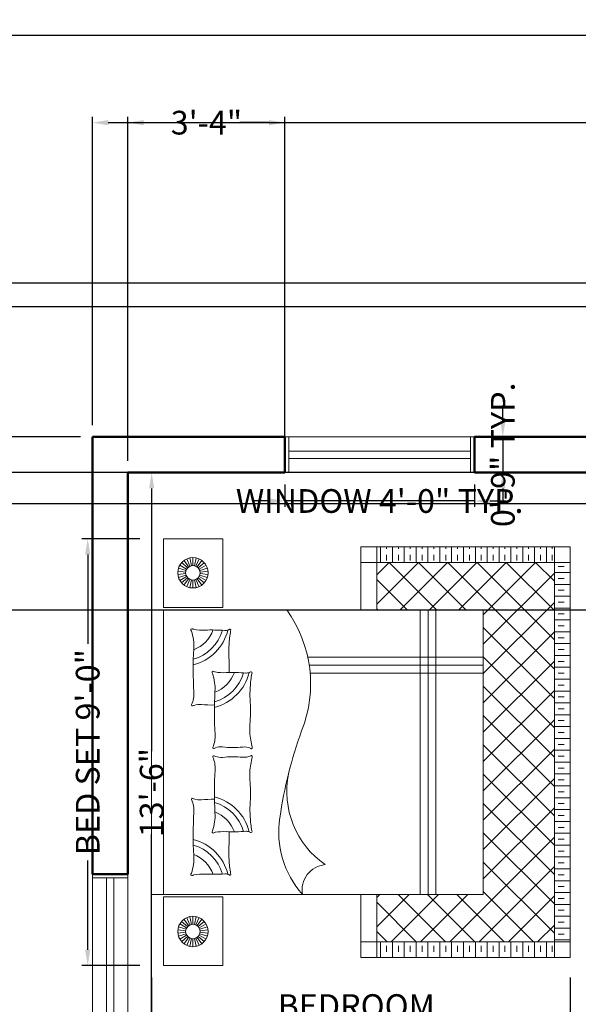
# Model space of a CAD drawing. Units: inches. Extents: x 6704 to 7574, y 11759 to 12617.
# Tile 6 of 8: x 6900 to 7041, y 12368 to 12617. Entities that reach past the tile are written whole.
import ezdxf

# ---------------------------------------------------------------- set-up
doc = ezdxf.new("R2010")
doc.units = ezdxf.units.IN
doc.header["$MEASUREMENT"] = 0
for name, color, linetype, lineweight in [('A-AREA-IDEN', 7, 'Continuous', 18), ('A-FURN', 8, 'Continuous', 18), ('C-PROP', 7, 'Continuous', 30), ('WALL', 7, 'Continuous', 50), ('WINDOW', 2, 'Continuous', 20), ('YQ_DIM', 3, 'Continuous', 18)]:
    doc.layers.add(name, color=color, linetype=linetype, lineweight=lineweight)
doc.styles.get("Standard").update_dxf_attribs({"font": 'arial.ttf'})
doc.styles.add('YQ_DIM', font='SUPEROS.SHX', dxfattribs={"width": 0.8, "bigfont": 'HZDX.SHX'})
doc.dimstyles.new('yqi0', dxfattribs={"dimscale": 0, "dimtxt": 6, "dimasz": 4, "dimexe": 1.5, "dimexo": 3, "dimgap": 0.5, "dimtad": 0, "dimdsep": 46, "dimlunit": 4, "dimtxsty": 'Standard', "dimcen": 0, "dimclrd": 256, "dimclre": 256, "dimclrt": 7, "dimadec": 1, "dimazin": 2, "dimtfac": 1, "dimtix": 1, "dimtmove": 2, "dimatfit": 2, "dimfxl": 1, "dimtolj": 1, "dimtzin": 0, "dimarcsym": 0})

# ---------------------------------------------------------------- blocks, each defined once
blk = doc.blocks.new('*D2')
at = {"layer": 'Defpoints', "color": 0, "transparency": 16777216}
for p in [(7311.07, 12612.93), (6879.07, 12550.26), (7311.07, 12550.26)]:
    blk.add_point(p, dxfattribs=at)
at = {"layer": 'YQ_DIM', "color": 0, "lineweight": -2, "transparency": 16777216}
for p, q in [((6879.07, 12553.26), (6879.07, 12614.43)), ((7311.07, 12553.26), (7311.07, 12614.43)), ((6883.07, 12612.93), (7089.48, 12612.93)), ((7307.07, 12612.93), (7100.66, 12612.93))]:
    blk.add_line(p, q, dxfattribs=at)
at = {"layer": 'YQ_DIM', "color": 0, "transparency": 16777216}
for points in [[(6883.07, 12613.6), (6883.07, 12612.27), (6879.07, 12612.93)], [(7307.07, 12613.6), (7307.07, 12612.27), (7311.07, 12612.93)]]:
    blk.add_solid(points, dxfattribs=at)
at = {"layer": 'YQ_DIM', "color": 0, "transparency": 16777216, "insert": (7095.07, 12612.93), "char_height": 6, "attachment_point": 5}
blk.add_mtext("\\A1;36'", dxfattribs=at)
blk = doc.blocks.new('*D4')
at = {"layer": 'Defpoints', "color": 0, "transparency": 16777216}
for p in [(6927.07, 12502.26), (6927.07, 12340.26), (6933.07, 12340.26)]:
    blk.add_point(p, dxfattribs=at)
at = {"layer": 'YQ_DIM', "color": 0, "lineweight": -2, "transparency": 16777216}
for p, q in [((6930.07, 12502.26), (6934.57, 12502.26)), ((6933.07, 12498.26), (6933.07, 12431.78)), ((6933.07, 12344.26), (6933.07, 12410.73)), ((6930.07, 12340.26), (6934.57, 12340.26))]:
    blk.add_line(p, q, dxfattribs=at)
at = {"layer": 'YQ_DIM', "color": 0, "transparency": 16777216}
for points in [[(6932.41, 12498.26), (6933.74, 12498.26), (6933.07, 12502.26)], [(6932.41, 12344.26), (6933.74, 12344.26), (6933.07, 12340.26)]]:
    blk.add_solid(points, dxfattribs=at)
at = {"layer": 'YQ_DIM', "color": 0, "transparency": 16777216, "insert": (6933.07, 12421.26), "char_height": 6, "attachment_point": 5, "rotation": 90}
blk.add_mtext('\\A1;13\'-6"', dxfattribs=at)
blk = doc.blocks.new('WD_00_X1')
for p, q in [((-0.5, 0.5), (0.5, 0.5)), ((-0.48, 0.5), (-0.48, -0.5)), ((0.48, 0.5), (0.48, -0.5)), ((0.48, 0.1), (-0.48, 0.1)), ((0.48, -0.1), (-0.48, -0.1)), ((-0.5, -0.5), (0.5, -0.5))]:
    blk.add_line(p, q)
blk = doc.blocks.new('BED')
h = blk.add_hatch()
h.set_pattern_fill('TRANS', color=256, scale=12, style=0)
h.set_pattern_definition([(360, (4433.967, -9715.0492), (1e-15, 3), []), (360, (4433.967, -9713.5492), (1e-15, 3), [1.5, -1.5])])
h.paths.add_polyline_path([(48, -103), (52, -103), (52, -58), (48, -58)])
h.paths.add_polyline_path([(-48, -58), (-52, -58), (-52, -103), (-48, -103)])
h = blk.add_hatch()
h.set_pattern_fill('ANSI37', color=256, scale=42, angle=-90, style=0)
h.set_pattern_definition([(315, (7787.1367, 4477.8466), (3.7123106, 3.7123106), []), (45, (7787.1367, 4477.8466), (-3.7123106, 3.7123106), [])])
h.paths.add_polyline_path([(-36, -85), (-36, -58), (-48, -58), (-48, -103), (48, -103), (48, -58), (36, -58), (36, -85)])
h = blk.add_hatch()
h.set_pattern_fill('TRANS', color=256, scale=12, angle=-90, style=0)
h.set_pattern_definition([(270, (4433.967, -9715.0492), (3, -1e-15), []), (270, (4435.467, -9715.0492), (3, -1e-15), [1.5, -1.5])])
h.paths.add_polyline_path([(48, -107), (48, -103), (-48, -103), (-48, -107)])
for p, q in [((-36, -1), (36, -1)), ((-36, -85), (-36, -1)), ((36, -1), (36, -85)), ((-54, -4), (-54, -19)), ((-36.64, -4), (-54, -4)), ((-36.64, -4), (-36.64, -19)), ((-36, -4), (36, -4)), ((36.64, -4), (36.64, -19)), ((36.64, -4), (54, -4)), ((54, -4), (54, -19)), ((-47.07, -10.7), (-48.9, -9.89)), ((-46.88, -10.37), (-48.5, -9.2)), ((-46.62, -10.08), (-47.96, -8.6)), ((-46.31, -9.86), (-47.31, -8.13)), ((-45.96, -9.7), (-46.58, -7.8)), ((-45.58, -9.62), (-45.8, -7.63)), ((-45.2, -9.62), (-45, -7.63)), ((-44.82, -9.7), (-44.21, -7.79)), ((-44.47, -9.85), (-43.48, -8.12)), ((-44.16, -10.08), (-42.83, -8.59)), ((-43.9, -10.36), (-42.29, -9.18)), ((-43.71, -10.7), (-41.89, -9.88)), ((43.71, -10.7), (41.89, -9.88)), ((43.9, -10.36), (42.29, -9.18)), ((44.16, -10.08), (42.83, -8.59)), ((44.47, -9.85), (43.48, -8.12)), ((44.82, -9.7), (44.21, -7.79)), ((45.2, -9.62), (45, -7.63)), ((45.58, -9.62), (45.8, -7.63)), ((45.96, -9.7), (46.58, -7.8)), ((46.31, -9.86), (47.31, -8.13)), ((46.62, -10.08), (47.96, -8.6)), ((46.88, -10.37), (48.5, -9.2)), ((47.07, -10.7), (48.9, -9.89)), ((-47.23, -11.45), (-49.23, -11.45)), ((-47.19, -11.07), (-49.14, -10.66)), ((-47.19, -11.83), (-49.14, -12.25)), ((-47.07, -12.2), (-48.89, -13.01)), ((-43.71, -12.19), (-41.88, -13)), ((-43.59, -11.06), (-41.64, -10.64)), ((-43.59, -11.83), (-41.63, -12.24)), ((-43.55, -11.44), (-41.55, -11.44)), ((43.55, -11.44), (41.55, -11.44)), ((43.59, -11.83), (41.63, -12.24)), ((43.59, -11.06), (41.64, -10.64)), ((43.71, -12.19), (41.88, -13)), ((47.07, -12.2), (48.89, -13.01)), ((47.19, -11.07), (49.14, -10.66)), ((47.19, -11.83), (49.14, -12.25)), ((47.23, -11.45), (49.23, -11.45)), ((-46.87, -12.53), (-48.49, -13.71)), ((-46.62, -12.81), (-47.95, -14.3)), ((-46.3, -13.04), (-47.3, -14.77)), ((-45.95, -13.2), (-46.57, -15.1)), ((-45.58, -13.27), (-45.78, -15.26)), ((-45.19, -13.27), (-44.98, -15.26)), ((-44.82, -13.19), (-44.2, -15.09)), ((-44.47, -13.04), (-43.46, -14.77)), ((-44.16, -12.81), (-42.82, -14.29)), ((-43.9, -12.52), (-42.28, -13.7)), ((43.9, -12.52), (42.28, -13.7)), ((44.16, -12.81), (42.82, -14.29)), ((44.47, -13.04), (43.46, -14.77)), ((44.82, -13.19), (44.2, -15.09)), ((45.19, -13.27), (44.98, -15.26)), ((45.58, -13.27), (45.78, -15.26)), ((45.95, -13.2), (46.57, -15.1)), ((46.3, -13.04), (47.3, -14.77)), ((46.62, -12.81), (47.95, -14.3)), ((46.87, -12.53), (48.49, -13.71)), ((-36.64, -19), (-54, -19)), ((36.64, -19), (54, -19)), ((20, -85), (20, -41.14)), ((22, -85), (22, -40.91)), ((24, -85), (24, -40.55)), ((-52, -54), (-52, -107)), ((-52, -54), (-36, -54)), ((-48, -54), (-48, -107)), ((36, -54), (52, -54)), ((48, -54), (48, -107)), ((52, -54), (52, -107)), ((-52, -58), (-36, -58)), ((36, -58), (52, -58)), ((36, -69), (-36, -69)), ((36, -71), (-36, -71)), ((36, -73), (-36, -73)), ((36, -85), (-36, -85)), ((-52, -103), (52, -103)), ((-52, -107), (52, -107))]:
    blk.add_line(p, q)
for centre, radius in [((-45.39, -11.45), 3.84), ((-45.39, -11.45), 1.84), ((45.39, -11.45), 3.84), ((45.39, -11.45), 1.84)]:
    blk.add_circle(centre, radius)
for centre, radius, start, end in [((-30.92, -11.24), 0.328, 35.8976, 208.6272), ((-42.38, -17.5), 12.73, 27.1629, 28.6272), ((-44.37, -13.89), 13.5, 357.4804, 9.3956), ((-33.8, -8.61), 8.46, 289.8695, 338.9843), ((-33.8, -8.61), 12.06, 283.8498, 346.0842), ((-33.8, -8.61), 10.71, 286.0319, 344.1205), ((-26.84, 0.13), 11.82, 251.1782, 273.3982), ((-20.92, -99.64), 88.13, 86.2964, 93.3982), ((-14.79, -4.98), 6.73, 266.2964, 294.303), ((-8.24, -13.16), 3.86, 159.0146, 186.273), ((-11.92, -11.33), 0.242, 335.7259, 114.303), ((-5.69, -14.14), 6.59, 155.7259, 159.0146), ((11.92, -11.33), 0.242, 65.697, 204.2741), ((5.69, -14.14), 6.59, 20.9854, 24.2741), ((8.24, -13.16), 3.86, 353.727, 20.9854), ((14.79, -4.98), 6.73, 245.697, 273.7036), ((20.92, -99.64), 88.13, 86.6018, 93.7036), ((33.8, -8.61), 12.06, 193.9158, 256.1502), ((33.8, -8.61), 10.71, 195.8795, 253.9681), ((33.8, -8.61), 8.46, 201.0157, 250.1305), ((26.84, 0.13), 11.82, 266.6018, 288.8218), ((30.92, -11.24), 0.328, 331.3728, 144.1024), ((44.37, -13.89), 13.5, 170.6044, 182.5196), ((42.38, -17.5), 12.73, 151.3728, 152.8371), ((10.15, -16.29), 41.07, 177.4804, 184.5075), ((-36.64, -16.28), 24.71, 358.5721, 6.273), ((36.64, -16.28), 24.71, 173.727, 181.4279), ((-10.15, -16.29), 41.07, 355.4925, 2.5196), ((-20.16, -16.62), 0.328, 35.8976, 208.6272), ((-31.62, -22.87), 12.73, 27.1629, 28.6272), ((-33.61, -19.26), 13.5, 357.4804, 9.3956), ((-23.04, -13.99), 8.46, 289.8695, 338.9843), ((-23.04, -13.99), 12.06, 283.8498, 346.0842), ((-23.04, -13.99), 10.71, 286.0319, 344.1205), ((-16.08, -5.24), 11.82, 251.1782, 273.3982), ((-10.15, -105.01), 88.13, 86.2964, 93.3982), ((-4.03, -10.35), 6.73, 266.2964, 294.303), ((2.52, -18.53), 3.86, 159.0146, 186.273), ((-1.16, -16.7), 0.242, 335.7259, 114.303), ((5.07, -19.51), 6.59, 155.7259, 159.0146), ((1.16, -16.7), 0.242, 65.697, 204.2741), ((-5.07, -19.51), 6.59, 20.9854, 24.2741), ((-2.52, -18.53), 3.86, 353.727, 20.9854), ((4.03, -10.35), 6.73, 245.697, 273.7036), ((10.15, -105.01), 88.13, 86.6018, 93.7036), ((23.04, -13.99), 12.06, 193.9158, 256.1502), ((23.04, -13.99), 10.71, 195.8795, 253.9681), ((23.04, -13.99), 8.46, 201.0157, 250.1305), ((16.08, -5.24), 11.82, 266.6018, 288.8218), ((20.16, -16.62), 0.328, 331.3728, 144.1024), ((33.61, -19.26), 13.5, 170.6044, 182.5196), ((31.62, -22.87), 12.73, 151.3728, 152.8371), ((-32.67, -19.67), 1.88, 339.2246, 4.5075), ((20.91, -21.66), 41.07, 177.4804, 184.5075), ((-25.88, -21.66), 24.71, 354.3784, 6.273), ((25.88, -21.66), 24.71, 173.727, 185.6216), ((-20.91, -21.66), 41.07, 355.4925, 2.5196), ((32.67, -19.67), 1.88, 175.4925, 200.7754), ((-30.88, -20.82), 0.25, 147.6219, 311.9343), ((-32.72, -19.65), 1.93, 327.6219, 339.2246), ((-25.16, -53.53), 33, 93.5164, 99.6766), ((-25.27, -51.86), 31.33, 86.4836, 93.5164), ((-21.12, 15.68), 36.34, 266.4836, 271.5234), ((21.12, 15.68), 36.34, 268.4766, 273.5164), ((25.27, -51.86), 31.33, 86.4836, 93.5164), ((25.16, -53.53), 33, 80.3234, 86.4836), ((30.88, -20.82), 0.25, 228.0657, 32.3781), ((32.72, -19.65), 1.93, 200.7754, 212.3781), ((-21.91, -25.04), 1.88, 339.2246, 4.5075), ((2.55, -24.46), 3.86, 174.3784, 204.7617), ((-2.55, -24.46), 3.86, 335.2383, 5.6216), ((21.91, -25.04), 1.88, 175.4925, 200.7754), ((-20.12, -26.19), 0.25, 147.6219, 311.9343), ((-21.96, -25.02), 1.93, 327.6219, 339.2246), ((-14.4, -58.9), 33, 93.5164, 99.6766), ((-14.51, -57.23), 31.33, 86.4836, 93.5164), ((-10.35, 10.3), 36.34, 266.4836, 275.306), ((-5.78, -38.98), 13.15, 77.9645, 95.306), ((2.5, -0.17), 26.53, 257.9645, 261.9243), ((-1.09, -26.25), 0.228, 231.9005, 52.8902), ((1.09, -26.25), 0.228, 127.1098, 308.0995), ((-2.5, -0.17), 26.53, 278.0757, 282.0355), ((5.78, -38.98), 13.15, 84.694, 102.0355), ((10.35, 10.3), 36.34, 264.694, 273.5164), ((14.51, -57.23), 31.33, 86.4836, 93.5164), ((14.4, -58.9), 33, 80.3234, 86.4836), ((20.12, -26.19), 0.25, 228.0657, 32.3781), ((21.96, -25.02), 1.93, 200.7754, 212.3781), ((-20.27, -56.85), 23.66, 81.0857, 131.6581), ((-32.56, -143.87), 111.55, 70.0977, 81.7735), ((-9.91, -57.83), 22.61, 78.6456, 145.1521), ((17.27, -9.21), 32.05, 248.2778, 305.7663), ((-34.97, -45.63), 6.55, 6.3172, 99.0807)]:
    blk.add_arc(centre, radius, start, end)
blk = doc.blocks.new('*D31')
at = {"layer": 'Defpoints', "color": 0, "transparency": 16777216}
for p in [(6966.82, 12502.26), (7014.82, 12502.26), (6966.82, 12495.06)]:
    blk.add_point(p, dxfattribs=at)
at = {"layer": 'YQ_DIM', "lineweight": -2, "transparency": 16777216}
for p, q in [((6966.82, 12499.26), (6966.82, 12493.56)), ((7014.82, 12499.26), (7014.82, 12493.56)), ((6962.82, 12495.06), (6958.82, 12495.06)), ((7014.82, 12495.06), (6966.82, 12495.06)), ((7018.82, 12495.06), (7022.82, 12495.06))]:
    blk.add_line(p, q, dxfattribs=at)
at = {"layer": 'YQ_DIM', "transparency": 16777216}
for points in [[(6962.82, 12495.72), (6962.82, 12494.39), (6966.82, 12495.06)], [(7018.82, 12495.72), (7018.82, 12494.39), (7014.82, 12495.06)]]:
    blk.add_solid(points, dxfattribs=at)
at = {"layer": 'YQ_DIM', "color": 7, "transparency": 16777216, "insert": (6990.82, 12495.06), "char_height": 6, "attachment_point": 5}
blk.add_mtext('\\A1;WINDOW 4\'-0" TYP.', dxfattribs=at)
blk = doc.blocks.new('*D32')
at = {"layer": 'Defpoints', "color": 0, "transparency": 16777216}
for p in [(7014.82, 12511.26), (7014.82, 12502.26), (7022.02, 12502.26)]:
    blk.add_point(p, dxfattribs=at)
at = {"layer": 'YQ_DIM', "lineweight": -2, "transparency": 16777216}
for p, q in [((7022.02, 12515.26), (7022.02, 12519.26)), ((7017.82, 12511.26), (7023.52, 12511.26)), ((7022.02, 12511.26), (7022.02, 12502.26)), ((7017.82, 12502.26), (7023.52, 12502.26)), ((7022.02, 12498.26), (7022.02, 12494.26))]:
    blk.add_line(p, q, dxfattribs=at)
at = {"layer": 'YQ_DIM', "transparency": 16777216}
for points in [[(7021.36, 12515.26), (7022.69, 12515.26), (7022.02, 12511.26)], [(7021.36, 12498.26), (7022.69, 12498.26), (7022.02, 12502.26)]]:
    blk.add_solid(points, dxfattribs=at)
at = {"layer": 'YQ_DIM', "color": 7, "transparency": 16777216, "insert": (7022.02, 12506.76), "char_height": 6, "attachment_point": 5, "rotation": 90}
blk.add_mtext('\\A1;0\'-9" TYP.', dxfattribs=at)
blk = doc.blocks.new('*D39')
at = {"layer": 'Defpoints', "color": 0, "transparency": 16777216}
for p in [(6916.87, 12485.5), (6933.07, 12485.5), (6933.07, 12377.5)]:
    blk.add_point(p, dxfattribs=at)
at = {"layer": 'YQ_DIM', "lineweight": -2, "transparency": 16777216}
for p, q in [((6930.07, 12485.5), (6915.37, 12485.5)), ((6916.87, 12481.5), (6916.87, 12458.93)), ((6916.87, 12381.5), (6916.87, 12404.06)), ((6930.07, 12377.5), (6915.37, 12377.5))]:
    blk.add_line(p, q, dxfattribs=at)
at = {"layer": 'YQ_DIM', "transparency": 16777216}
for points in [[(6916.21, 12481.5), (6917.54, 12481.5), (6916.87, 12485.5)], [(6916.21, 12381.5), (6917.54, 12381.5), (6916.87, 12377.5)]]:
    blk.add_solid(points, dxfattribs=at)
at = {"layer": 'YQ_DIM', "color": 7, "transparency": 16777216, "insert": (6916.87, 12431.5), "char_height": 6, "attachment_point": 5, "rotation": 90}
blk.add_mtext('\\A1;BED SET 9\'-0"', dxfattribs=at)
blk = doc.blocks.new('*D40')
at = {"layer": 'Defpoints', "color": 0, "transparency": 16777216}
for p in [(6933.07, 12377.5), (7039.07, 12377.5), (6933.07, 12361.3)]:
    blk.add_point(p, dxfattribs=at)
at = {"layer": 'YQ_DIM', "lineweight": -2, "transparency": 16777216}
for p, q in [((6933.07, 12374.5), (6933.07, 12359.8)), ((7039.07, 12374.5), (7039.07, 12359.8)), ((6937.07, 12361.3), (6975.26, 12361.3)), ((7035.07, 12361.3), (6996.88, 12361.3))]:
    blk.add_line(p, q, dxfattribs=at)
at = {"layer": 'YQ_DIM', "transparency": 16777216}
for points in [[(6937.07, 12361.96), (6937.07, 12360.63), (6933.07, 12361.3)], [(7035.07, 12361.96), (7035.07, 12360.63), (7039.07, 12361.3)]]:
    blk.add_solid(points, dxfattribs=at)
at = {"layer": 'YQ_DIM', "color": 7, "transparency": 16777216, "insert": (6986.07, 12361.3), "char_height": 6, "attachment_point": 5}
blk.add_mtext('\\A1;8\'-10"', dxfattribs=at)
blk = doc.blocks.new('*D55')
at = {"layer": 'Defpoints', "color": 0, "transparency": 16777216}
for p in [(7269.07, 12590.81), (6918.07, 12511.26), (7269.07, 12511.26)]:
    blk.add_point(p, dxfattribs=at)
at = {"layer": 'YQ_DIM', "lineweight": -2, "transparency": 16777216}
for p, q in [((6918.07, 12514.26), (6918.07, 12592.31)), ((7269.07, 12514.26), (7269.07, 12592.31)), ((6922.07, 12590.81), (7082.72, 12590.81)), ((7265.07, 12590.81), (7104.43, 12590.81))]:
    blk.add_line(p, q, dxfattribs=at)
at = {"layer": 'YQ_DIM', "transparency": 16777216}
for points in [[(6922.07, 12591.47), (6922.07, 12590.14), (6918.07, 12590.81)], [(7265.07, 12591.47), (7265.07, 12590.14), (7269.07, 12590.81)]]:
    blk.add_solid(points, dxfattribs=at)
at = {"layer": 'YQ_DIM', "color": 7, "transparency": 16777216, "insert": (7093.57, 12590.81), "char_height": 6, "attachment_point": 5}
blk.add_mtext('\\A1;29\'-3"', dxfattribs=at)
blk = doc.blocks.new('*D56')
at = {"layer": 'Defpoints', "color": 0, "transparency": 16777216}
for p in [(6712.97, 12511.26), (6918.07, 12511.26), (6918.07, 12011.76)]:
    blk.add_point(p, dxfattribs=at)
at = {"layer": 'YQ_DIM', "lineweight": -2, "transparency": 16777216}
for p, q in [((6915.07, 12511.26), (6711.47, 12511.26)), ((6712.97, 12507.26), (6712.97, 12279.42)), ((6712.97, 12015.76), (6712.97, 12243.59)), ((6915.07, 12011.76), (6711.47, 12011.76))]:
    blk.add_line(p, q, dxfattribs=at)
at = {"layer": 'YQ_DIM', "transparency": 16777216}
for points in [[(6712.3, 12507.26), (6713.64, 12507.26), (6712.97, 12511.26)], [(6712.3, 12015.76), (6713.64, 12015.76), (6712.97, 12011.76)]]:
    blk.add_solid(points, dxfattribs=at)
at = {"layer": 'YQ_DIM', "color": 7, "transparency": 16777216, "insert": (6712.97, 12261.51), "char_height": 6, "attachment_point": 5, "rotation": 90}
blk.add_mtext('\\A1;41\'-7 1/2"', dxfattribs=at)
blk = doc.blocks.new('*D57')
at = {"layer": 'Defpoints', "color": 0, "transparency": 16777216}
for p in [(6879.07, 12550.26), (6712.97, 12511.26), (6918.07, 12511.26)]:
    blk.add_point(p, dxfattribs=at)
at = {"layer": 'YQ_DIM', "lineweight": -2, "transparency": 16777216}
for p, q in [((6876.07, 12550.26), (6711.47, 12550.26)), ((6712.97, 12546.26), (6712.97, 12539.23)), ((6712.97, 12515.26), (6712.97, 12522.28)), ((6915.07, 12511.26), (6711.47, 12511.26))]:
    blk.add_line(p, q, dxfattribs=at)
at = {"layer": 'YQ_DIM', "transparency": 16777216}
for points in [[(6712.3, 12546.26), (6713.64, 12546.26), (6712.97, 12550.26)], [(6712.3, 12515.26), (6713.64, 12515.26), (6712.97, 12511.26)]]:
    blk.add_solid(points, dxfattribs=at)
at = {"layer": 'YQ_DIM', "color": 7, "transparency": 16777216, "insert": (6712.97, 12530.76), "char_height": 6, "attachment_point": 5, "rotation": 90}
blk.add_mtext('\\A1;3\'-3"', dxfattribs=at)
blk = doc.blocks.new('*D75')
at = {"layer": 'Defpoints', "color": 0, "transparency": 16777216}
for p in [(6966.82, 12590.81), (6927.07, 12502.26), (6966.82, 12502.26)]:
    blk.add_point(p, dxfattribs=at)
at = {"layer": 'YQ_DIM', "lineweight": -2, "transparency": 16777216}
for p, q in [((6927.07, 12505.26), (6927.07, 12592.31)), ((6966.82, 12505.26), (6966.82, 12592.31)), ((6931.07, 12590.81), (6938.47, 12590.81)), ((6962.82, 12590.81), (6955.42, 12590.81))]:
    blk.add_line(p, q, dxfattribs=at)
at = {"layer": 'YQ_DIM', "transparency": 16777216}
for points in [[(6931.07, 12591.47), (6931.07, 12590.14), (6927.07, 12590.81)], [(6962.82, 12591.47), (6962.82, 12590.14), (6966.82, 12590.81)]]:
    blk.add_solid(points, dxfattribs=at)
at = {"layer": 'YQ_DIM', "color": 7, "transparency": 16777216, "insert": (6946.95, 12590.81), "char_height": 6, "attachment_point": 5}
blk.add_mtext('\\A1;3\'-4"', dxfattribs=at)
blk = doc.blocks.new('*D76')
at = {"layer": 'Defpoints', "color": 0, "transparency": 16777216}
for p in [(7260.07, 12502.26), (6712.97, 12467.43), (7260.07, 12467.43)]:
    blk.add_point(p, dxfattribs=at)
at = {"layer": 'YQ_DIM', "lineweight": -2, "transparency": 16777216}
for p, q in [((7257.07, 12502.26), (6711.47, 12502.26)), ((6712.97, 12498.26), (6712.97, 12495.7)), ((6712.97, 12471.43), (6712.97, 12473.99)), ((7257.07, 12467.43), (6711.47, 12467.43))]:
    blk.add_line(p, q, dxfattribs=at)
at = {"layer": 'YQ_DIM', "transparency": 16777216}
for points in [[(6712.3, 12498.26), (6713.64, 12498.26), (6712.97, 12502.26)], [(6712.3, 12471.43), (6713.64, 12471.43), (6712.97, 12467.43)]]:
    blk.add_solid(points, dxfattribs=at)
at = {"layer": 'YQ_DIM', "color": 7, "transparency": 16777216, "insert": (6712.97, 12484.84), "char_height": 6, "attachment_point": 5, "rotation": 90}
blk.add_mtext('\\A1;2\'-11"', dxfattribs=at)
blk = doc.blocks.new('*D81')
at = {"layer": 'Defpoints', "color": 0, "transparency": 16777216}
for p in [(7063.57, 12502.26), (6712.97, 12494.38), (7063.57, 12494.38)]:
    blk.add_point(p, dxfattribs=at)
at = {"layer": 'YQ_DIM', "lineweight": -2, "transparency": 16777216}
for p, q in [((6712.97, 12506.26), (6712.97, 12510.26)), ((7060.57, 12502.26), (6711.47, 12502.26)), ((6712.97, 12502.26), (6712.97, 12494.38)), ((7060.57, 12494.38), (6711.47, 12494.38)), ((6712.97, 12490.38), (6712.97, 12486.38))]:
    blk.add_line(p, q, dxfattribs=at)
at = {"layer": 'YQ_DIM', "transparency": 16777216}
for points in [[(6712.3, 12506.26), (6713.64, 12506.26), (6712.97, 12502.26)], [(6712.3, 12490.38), (6713.64, 12490.38), (6712.97, 12494.38)]]:
    blk.add_solid(points, dxfattribs=at)
at = {"layer": 'YQ_DIM', "color": 7, "transparency": 16777216, "insert": (6712.97, 12498.32), "char_height": 6, "attachment_point": 5, "rotation": 90}
blk.add_mtext('\\A1;0\'-8"', dxfattribs=at)

msp = doc.modelspace()

# ---------------------------------------------------------------- linework, layer by layer
at = {"layer": 'C-PROP'}
for p, q in [((6879.073, 12550.257), (7311.073, 12550.257)), ((6885.073, 12544.257), (7305.073, 12544.257))]:
    msp.add_line(p, q, dxfattribs=at)
at = {"layer": 'WALL'}
for p, q in [((6918.073, 12511.257), (6966.823, 12511.257)), ((6918.073, 12400.631), (6918.073, 12511.257)), ((6966.823, 12502.257), (6966.823, 12511.257)), ((7014.823, 12511.257), (7054.573, 12511.257)), ((7014.823, 12502.257), (7014.823, 12511.257)), ((6927.073, 12502.257), (6966.823, 12502.257)), ((6927.073, 12400.631), (6927.073, 12502.257)), ((7014.823, 12502.257), (7054.573, 12502.257)), ((6927.073, 12400.631), (6918.073, 12400.631))]:
    msp.add_line(p, q, dxfattribs=at)

# ---------------------------------------------------------------- block references
at = {"layer": 'A-FURN', "rotation": 90}
msp.add_blockref('BED', (6932.073, 12431.496), dxfattribs=at)
at = {"layer": 'WINDOW', "xscale": 48, "zscale": 48}
for p, yscale, rotation in [((6990.823, 12506.757), 9, 180.0000000000021), ((6922.573, 12376.631), 8.99999999999909, 90)]:
    msp.add_blockref('WD_00_X1', p, dxfattribs=dict(at, yscale=yscale, rotation=rotation))

# ---------------------------------------------------------------- texts
at = {"layer": 'A-AREA-IDEN', "insert": (6969.109, 12370.233), "char_height": 13.77953, "width": 31.54746, "attachment_point": 1, "style": 'YQ_DIM'}
msp.add_mtext('\\pxqc;{\\H0.43543x;BEDROOM}', dxfattribs=at)

# ---------------------------------------------------------------- dimensions: what is measured, and where the dimension line sits
at = {"layer": 'YQ_DIM'}
dim = msp.add_aligned_dim(p1=(6879.073, 12550.257), p2=(7311.073, 12550.257), distance=62.676, dimstyle='yqi0', override={"dimscale": 1, "dimclrd": 0, "dimclre": 0, "dimclrt": 0}, dxfattribs=at)
dim.commit()
dim.dimension.update_dxf_attribs({"geometry": '*D2', "text_midpoint": (7095.073, 12612.934)})
for base, p1, p2, picture, middle in [((7269.073, 12590.807), (6918.073, 12511.257), (7269.073, 12511.257), '*D55', (7093.573, 12590.807)), ((6966.82251, 12590.80733), (6927.0725, 12502.25733), (6966.82251, 12502.25733), '*D75', (6946.94751, 12590.80733))]:
    dim = msp.add_linear_dim(base=base, p1=p1, p2=p2, dimstyle='yqi0', override={"dimscale": 1, "dimdec": 1, "dimzin": 1, "dimfrac": 2}, dxfattribs=at)
    dim.commit()
    dim.dimension.update_dxf_attribs({"geometry": picture, "text_midpoint": middle})
for base, p1, p2, angle, override, picture, middle in [((6712.97, 12511.257), (6879.073, 12550.257), (6918.073, 12511.257), 90, {"dimscale": 1, "dimdec": 1, "dimzin": 1, "dimfrac": 2}, '*D57', (6712.97, 12530.757)), ((6712.97, 12511.257), (6918.073, 12011.757), (6918.073, 12511.257), 90, {"dimscale": 1, "dimdec": 1, "dimzin": 1, "dimfrac": 2}, '*D56', (6712.97, 12261.507)), ((6712.97, 12494.383), (7063.573, 12502.257), (7063.573, 12494.383), 90, {"dimscale": 1, "dimdec": 1, "dimzin": 1, "dimfrac": 2}, '*D81', (6712.97, 12498.32)), ((6712.97, 12467.428), (7260.073, 12502.257), (7260.073, 12467.428), 90, {"dimscale": 1, "dimdec": 1, "dimzin": 1, "dimfrac": 2}, '*D76', (6712.97, 12484.842)), ((6933.073, 12340.257), (6927.073, 12502.257), (6927.073, 12340.257), 270, {"dimscale": 1, "dimclrd": 0, "dimclre": 0, "dimclrt": 0}, '*D4', (6933.073, 12421.257)), ((6933.073, 12361.296), (7039.073, 12377.496), (6933.073, 12377.496), 180, {"dimscale": 1, "dimdec": 1, "dimzin": 1, "dimfrac": 2}, '*D40', (6986.073, 12361.296))]:
    dim = msp.add_linear_dim(base=base, p1=p1, p2=p2, angle=angle, dimstyle='yqi0', override=override, dxfattribs=at)
    dim.commit()
    dim.dimension.update_dxf_attribs({"geometry": picture, "text_midpoint": middle})
for base, p1, p2, angle, text, picture, middle in [((7022.023, 12502.257), (7014.823, 12511.257), (7014.823, 12502.257), 270, '<> TYP.', '*D32', (7022.023, 12506.757)), ((6966.823, 12495.057), (7014.823, 12502.257), (6966.823, 12502.257), 180, 'WINDOW <> TYP.', '*D31', (6990.823, 12495.057)), ((6916.873, 12485.496), (6933.073, 12377.496), (6933.073, 12485.496), 90, 'BED SET <>', '*D39', (6916.873, 12431.496))]:
    dim = msp.add_linear_dim(base=base, p1=p1, p2=p2, angle=angle, text=text, dimstyle='yqi0', override={"dimscale": 1, "dimdec": 1, "dimzin": 1, "dimfrac": 2}, dxfattribs=at)
    dim.commit()
    dim.dimension.update_dxf_attribs({"geometry": picture, "text_midpoint": middle})

doc.saveas('drawing.dxf')
